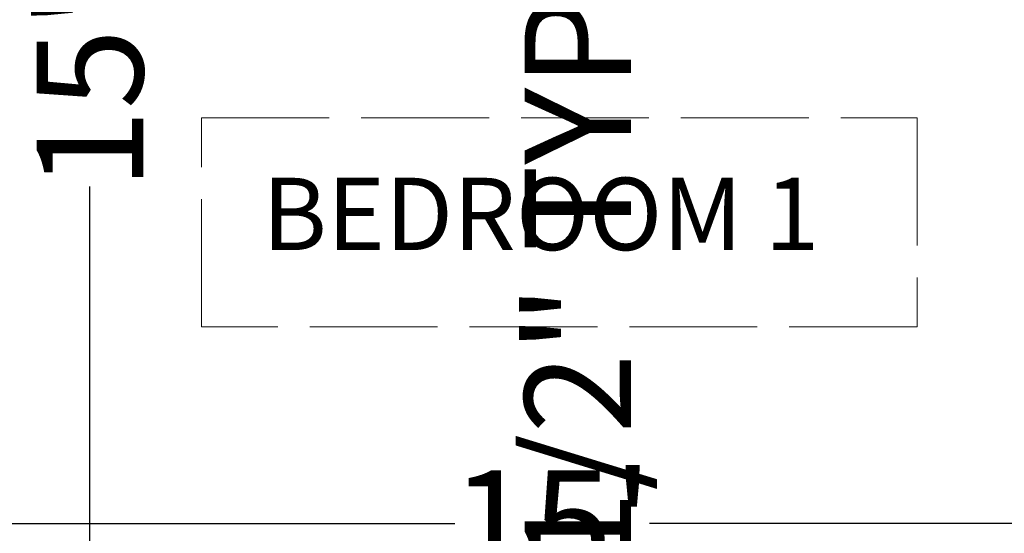
# Model space of a CAD drawing. Units: inches. Extents: x -269 to 4574, y -694 to 313.
# Tile 11 of 19: x 302 to 395, y -122 to -74. Entities that reach past the tile are written whole.
import ezdxf

# ---------------------------------------------------------------- set-up
doc = ezdxf.new("R2010")
doc.units = ezdxf.units.IN
doc.header["$MEASUREMENT"] = 0
doc.linetypes.add('ACAD_ISO02W100', pattern=[15, 12, -3])
for name, color, linetype, lineweight in [('A-ANNO-FRAM', 7, 'ACAD_ISO02W100', 13), ('A-AREA-IDEN', 6, 'Continuous', 20), ('DIMENSION', 5, 'Continuous', 18)]:
    doc.layers.add(name, color=color, linetype=linetype, lineweight=lineweight)
doc.dimstyles.get("Standard").update_dxf_attribs({"dimtxt": 10, "dimasz": 0.18, "dimexe": 0.18, "dimexo": 0.0625, "dimgap": 0.09, "dimtad": 0, "dimdec": 1, "dimzin": 0, "dimdsep": 46, "dimlunit": 3, "dimtxsty": 'Standard', "dimcen": 0.09, "dimclrt": 7, "dimadec": 0, "dimazin": 0, "dimtfac": 1, "dimtdec": 1, "dimtofl": 0, "dimtmove": 0, "dimatfit": 3, "dimfxl": 1, "dimtolj": 1, "dimtzin": 0, "dimarcsym": 0})

# ---------------------------------------------------------------- blocks, each defined once
blk = doc.blocks.new('*D19')
at = {"layer": 'Defpoints', "color": 0, "lineweight": 0, "transparency": 16777216}
for p in [(308.758, 9.268), (313.445, 9.268), (313.445, -170.732)]:
    blk.add_point(p, dxfattribs=at)
at = {"layer": 'DIMENSION', "color": 0, "lineweight": -2, "transparency": 16777216}
for p, q in [((313.383, 9.268), (308.578, 9.268)), ((308.758, 9.088), (308.758, -71.594)), ((308.758, -170.552), (308.758, -89.869)), ((313.383, -170.732), (308.578, -170.732))]:
    blk.add_line(p, q, dxfattribs=at)
at = {"layer": 'DIMENSION', "color": 0, "lineweight": 0, "transparency": 16777216}
for points in [[(308.728, 9.088), (308.788, 9.088), (308.758, 9.268)], [(308.728, -170.552), (308.788, -170.552), (308.758, -170.732)]]:
    blk.add_solid(points, dxfattribs=at)
at = {"layer": 'DIMENSION', "color": 0, "transparency": 16777216, "insert": (308.758, -80.732), "char_height": 10, "attachment_point": 5, "rotation": 90}
blk.add_mtext("\\A1;15'", dxfattribs=at)
blk = doc.blocks.new('*D20')
at = {"layer": 'Defpoints', "color": 0, "lineweight": 0, "transparency": 16777216}
for p in [(442.137, -121.555), (262.137, -122.439), (442.137, -122.439)]:
    blk.add_point(p, dxfattribs=at)
at = {"layer": 'DIMENSION', "color": 0, "lineweight": -2, "transparency": 16777216}
for p, q in [((262.137, -122.376), (262.137, -121.375)), ((262.317, -121.555), (342.999, -121.555)), ((441.957, -121.555), (361.275, -121.555)), ((442.137, -122.376), (442.137, -121.375))]:
    blk.add_line(p, q, dxfattribs=at)
at = {"layer": 'DIMENSION', "color": 0, "lineweight": 0, "transparency": 16777216}
for points in [[(262.317, -121.525), (262.317, -121.585), (262.137, -121.555)], [(441.957, -121.525), (441.957, -121.585), (442.137, -121.555)]]:
    blk.add_solid(points, dxfattribs=at)
at = {"layer": 'DIMENSION', "color": 0, "transparency": 16777216, "insert": (352.137, -121.555), "char_height": 10, "attachment_point": 5}
blk.add_mtext("\\A1;15'", dxfattribs=at)
blk = doc.blocks.new('*D49')
at = {"layer": 'Defpoints', "color": 0, "lineweight": 0, "transparency": 16777216}
for p in [(344.278, -221.793), (354.546, -221.793), (344.278, -290.244)]:
    blk.add_point(p, dxfattribs=at)
at = {"layer": 'DIMENSION', "color": 0, "lineweight": -2, "transparency": 16777216}
for p, q in [((354.546, -221.793), (354.546, -221.613)), ((344.34, -221.793), (354.726, -221.793)), ((354.546, -290.064), (354.546, -221.973)), ((344.34, -290.244), (354.726, -290.244))]:
    blk.add_line(p, q, dxfattribs=at)
at = {"layer": 'DIMENSION', "color": 0, "lineweight": 0, "transparency": 16777216}
for points in [[(354.516, -221.973), (354.576, -221.973), (354.546, -221.793)], [(354.516, -290.064), (354.576, -290.064), (354.546, -290.244)]]:
    blk.add_solid(points, dxfattribs=at)
at = {"layer": 'DIMENSION', "color": 7, "transparency": 16777216, "insert": (354.546, -133.666), "char_height": 10, "attachment_point": 5, "rotation": 90}
blk.add_mtext('\\A1;COVER 5\'-8 1/2" TYP.', dxfattribs=at)

msp = doc.modelspace()

# ---------------------------------------------------------------- linework, layer by layer
at = {"layer": 'A-ANNO-FRAM'}
msp.add_lwpolyline([(319.222, -83.425), (386.384, -83.425), (386.384, -103.078), (319.222, -103.078)], close=True, dxfattribs=at)

# ---------------------------------------------------------------- texts
at = {"layer": 'A-AREA-IDEN'}
msp.add_text('BEDROOM 1 ', height=6.7934, dxfattribs=at).set_placement((324.92, -95.855))

# ---------------------------------------------------------------- dimensions: what is measured, and where the dimension line sits
at = {"layer": 'DIMENSION'}
dim = msp.add_linear_dim(base=(308.758, 9.268), p1=(313.445, -170.732), p2=(313.445, 9.268), angle=90, dimstyle='Standard', override={"dimclrd": 0, "dimclre": 0, "dimclrt": 0}, dxfattribs=at)
dim.commit()
dim.dimension.update_dxf_attribs({"geometry": '*D19', "text_midpoint": (308.758, -80.732)})
dim = msp.add_linear_dim(base=(354.546, -221.793), p1=(344.278, -290.244), p2=(344.278, -221.793), angle=90, text='COVER <> TYP.', dimstyle='Standard', override={"dimdec": 1, "dimlfac": 1, "dimrnd": 0, "dimzin": 1, "dimdsep": 46, "dimlunit": 4, "dimfrac": 2}, dxfattribs=at)
dim.commit()
dim.dimension.update_dxf_attribs({"geometry": '*D49', "text_midpoint": (354.546, -133.666)})
dim = msp.add_linear_dim(base=(442.137, -121.555), p1=(262.137, -122.439), p2=(442.137, -122.439), dimstyle='Standard', override={"dimclrd": 0, "dimclre": 0, "dimclrt": 0}, dxfattribs=at)
dim.commit()
dim.dimension.update_dxf_attribs({"geometry": '*D20', "text_midpoint": (352.137, -121.555)})

doc.saveas('drawing.dxf')
